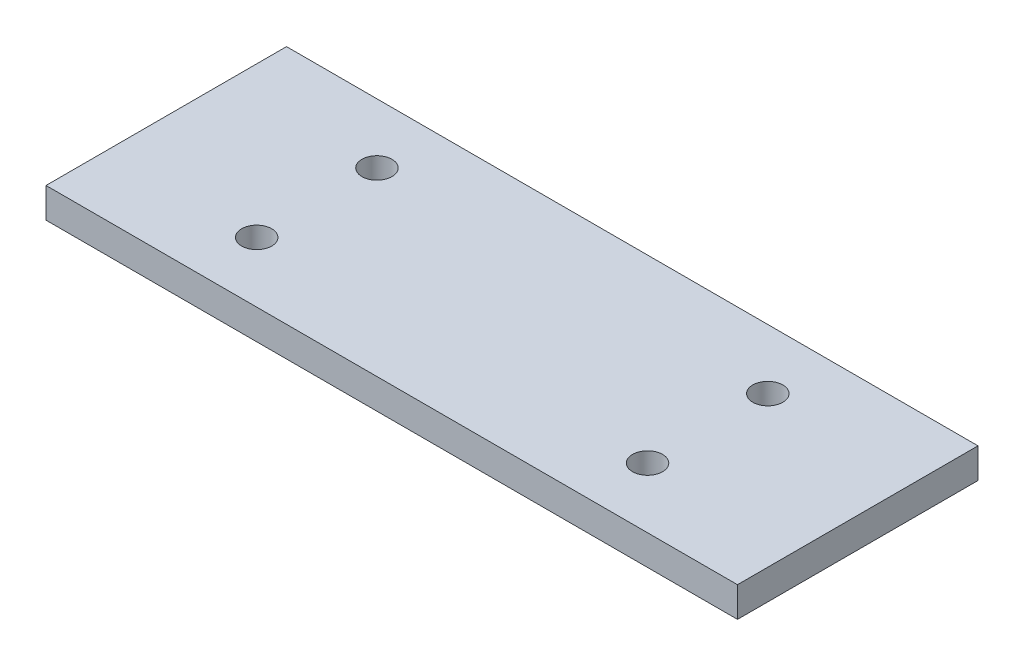
from build123d import *

# Parameters (mm, degrees)
BASE_PLATE_PROFILE_WITH_4_HOLES_W = 115
BASE_PLATE_PROFILE_WITH_4_HOLES_H = 40
BASE_PLATE_PROFILE_WITH_4_HOLES_R = 2.5
BASE_PLATE_115X40X5_DEPTH         = 5


with BuildPart() as part:
    # Base Plate Profile with 4 Holes → Base Plate 115x40x5 (new body)
    with BuildSketch(Plane(origin=(0, 0, 0), x_dir=(1, 0, 0), z_dir=(0, 1, 0))):
        Rectangle(BASE_PLATE_PROFILE_WITH_4_HOLES_W, BASE_PLATE_PROFILE_WITH_4_HOLES_H)
        with Locations(Location((-32.5, 10.041360294, 0), (0, 0, 270))):
            Circle(BASE_PLATE_PROFILE_WITH_4_HOLES_R, mode=Mode.SUBTRACT)
        with Locations(Location((-32.5, -9.958639706, 0), (0, 0, 270))):
            Circle(BASE_PLATE_PROFILE_WITH_4_HOLES_R, mode=Mode.SUBTRACT)
        with Locations(Location((32.5, -9.958639706, 0), (0, 0, 90))):
            Circle(BASE_PLATE_PROFILE_WITH_4_HOLES_R, mode=Mode.SUBTRACT)
        with Locations(Location((32.5, 10.041360294, 0), (0, 0, 90))):
            Circle(BASE_PLATE_PROFILE_WITH_4_HOLES_R, mode=Mode.SUBTRACT)
    extrude(amount=BASE_PLATE_115X40X5_DEPTH)


solid = part.part
